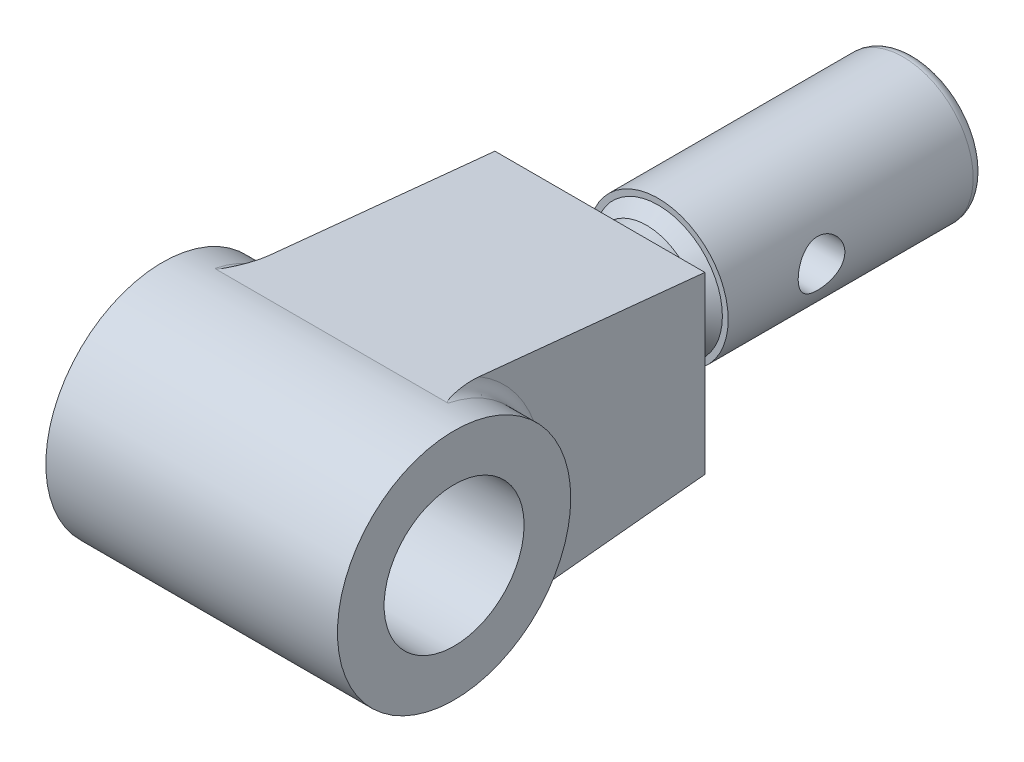
ISO-10303-21;
HEADER;
FILE_DESCRIPTION(('STEP AP214'),'2;1');
FILE_NAME('part.step','',(''),(''),'','','');
FILE_SCHEMA(('AUTOMOTIVE_DESIGN { 1 0 10303 214 1 1 1 1 }'));
ENDSEC;
DATA;
#1=APPLICATION_CONTEXT('core data for automotive mechanical design processes');
#2=APPLICATION_PROTOCOL_DEFINITION('international standard','automotive_design',2000,#1);
#3=PRODUCT_CONTEXT('',#1,'mechanical');
#4=PRODUCT('Part','Part','',(#3));
#5=PRODUCT_RELATED_PRODUCT_CATEGORY('part','',(#4));
#6=PRODUCT_DEFINITION_FORMATION('','',#4);
#7=PRODUCT_DEFINITION_CONTEXT('part definition',#1,'design');
#8=PRODUCT_DEFINITION('design','',#6,#7);
#9=PRODUCT_DEFINITION_SHAPE('','',#8);
#10=(LENGTH_UNIT() NAMED_UNIT(*) SI_UNIT(.MILLI.,.METRE.));
#11=(NAMED_UNIT(*) PLANE_ANGLE_UNIT() SI_UNIT($,.RADIAN.));
#12=(NAMED_UNIT(*) SI_UNIT($,.STERADIAN.) SOLID_ANGLE_UNIT());
#13=UNCERTAINTY_MEASURE_WITH_UNIT(LENGTH_MEASURE(1.E-05),#10,'distance_accuracy_value','');
#14=(GEOMETRIC_REPRESENTATION_CONTEXT(3) GLOBAL_UNCERTAINTY_ASSIGNED_CONTEXT((#13)) GLOBAL_UNIT_ASSIGNED_CONTEXT((#10,
#11,#12)) REPRESENTATION_CONTEXT('',''));
#15=CARTESIAN_POINT('',(0.,0.,0.));
#16=DIRECTION('',(0.,0.,1.));
#17=DIRECTION('',(1.,0.,0.));
#18=AXIS2_PLACEMENT_3D('',#15,#16,#17);
#19=CARTESIAN_POINT('',(0.,4.75247524752475,-0.475247524752475));
#20=DIRECTION('',(0.,0.995037190209989,-0.0995037190209989));
#21=DIRECTION('',(0.,0.0995037190209989,0.995037190209989));
#22=AXIS2_PLACEMENT_3D('',#19,#20,#21);
#23=PLANE('',#22);
#24=DIRECTION('',(0.,-0.0995037190209989,-0.995037190209989));
#25=VECTOR('',#24,1.);
#26=CARTESIAN_POINT('',(-9.,10.,52.));
#27=LINE('',#26,#25);
#28=CARTESIAN_POINT('',(-9.,9.43438132008126,46.3438132008126));
#29=VERTEX_POINT('',#28);
#30=CARTESIAN_POINT('',(-9.,7.5,27.));
#31=VERTEX_POINT('',#30);
#32=EDGE_CURVE('E120',#29,#31,#27,.T.);
#33=ORIENTED_EDGE('',*,*,#32,.F.);
#34=CARTESIAN_POINT('',(-9.,9.43438132008126,46.3438132008126));
#35=CARTESIAN_POINT('',(-9.00001459803866,9.44279857819186,46.4279857819186));
#36=CARTESIAN_POINT('',(-9.00195007259903,9.45121395233566,46.5121395233566));
#37=CARTESIAN_POINT('',(-9.00925721243809,9.46802699368894,46.6802699368894));
#38=CARTESIAN_POINT('',(-9.01462757621855,9.47642466639695,46.7642466639695));
#39=CARTESIAN_POINT('',(-9.02839065402064,9.4931839174512,46.931839174512));
#40=CARTESIAN_POINT('',(-9.03677945197559,9.50154552842399,47.0154552842398));
#41=CARTESIAN_POINT('',(-9.05626603490288,9.51823793957924,47.1823793957924));
#42=CARTESIAN_POINT('',(-9.06736410968055,9.52656873636875,47.2656873636875));
#43=CARTESIAN_POINT('',(-9.1042239175738,9.55145319834917,47.5145319834917));
#44=CARTESIAN_POINT('',(-9.13360055531106,9.5679543693951,47.679543693951));
#45=CARTESIAN_POINT('',(-9.20036560076197,9.60079627564721,48.0079627564722));
#46=CARTESIAN_POINT('',(-9.23775582627735,9.61713697357066,48.1713697357066));
#47=CARTESIAN_POINT('',(-9.30382525269167,9.64337755100343,48.4337755100343));
#48=CARTESIAN_POINT('',(-9.3303085460812,9.65333275535504,48.5333275535504));
#49=CARTESIAN_POINT('',(-9.38591969959388,9.6731705062701,48.7317050627009));
#50=CARTESIAN_POINT('',(-9.41504775619662,9.68305304737633,48.8305304737633));
#51=CARTESIAN_POINT('',(-9.4868107569843,9.70619439893835,49.0619439893834));
#52=CARTESIAN_POINT('',(-9.53059368398147,9.71941852182165,49.1941852182164));
#53=CARTESIAN_POINT('',(-9.6098255608624,9.74130040667283,49.4130040667283));
#54=CARTESIAN_POINT('',(-9.64327328731144,9.7500283022922,49.500283022922));
#55=CARTESIAN_POINT('',(-9.70409318445665,9.7644107399891,49.644107399891));
#56=CARTESIAN_POINT('',(-9.72984469495091,9.77013184956829,49.7013184956829));
#57=CARTESIAN_POINT('',(-9.77730952141487,9.77951878900499,49.7951878900499));
#58=CARTESIAN_POINT('',(-9.79763054155861,9.78325029234061,49.8325029234061));
#59=CARTESIAN_POINT('',(-9.83152593740173,9.788625396293,49.88625396293));
#60=CARTESIAN_POINT('',(-9.84336282293241,9.79037636611875,49.9037636611875));
#61=CARTESIAN_POINT('',(-9.86880656445889,9.79374682709678,49.9374682709678));
#62=CARTESIAN_POINT('',(-9.88240732968119,9.79536674089937,49.9536674089937));
#63=CARTESIAN_POINT('',(-9.90362979230834,9.7974453615268,49.974453615268));
#64=CARTESIAN_POINT('',(-9.91003887946058,9.79802485359438,49.9802485359437));
#65=CARTESIAN_POINT('',(-9.92347492697489,9.79911049653625,49.9911049653625));
#66=CARTESIAN_POINT('',(-9.93050194685285,9.79961664033359,49.9961664033359));
#67=CARTESIAN_POINT('',(-9.94390664000616,9.80043519672147,50.0043519672147));
#68=CARTESIAN_POINT('',(-9.95016816320597,9.80076611032304,50.0076611032304));
#69=CARTESIAN_POINT('',(-9.96313447059713,9.80132304768613,50.0132304768613));
#70=CARTESIAN_POINT('',(-9.96983721587579,9.80154951986671,50.015495198667));
#71=CARTESIAN_POINT('',(-9.98050267325267,9.80179749812321,50.017974981232));
#72=CARTESIAN_POINT('',(-9.98435828622742,9.8018653659966,50.018653659966));
#73=CARTESIAN_POINT('',(-9.99214094724413,9.80195700184466,50.0195700184466));
#74=CARTESIAN_POINT('',(-9.99606825420468,9.80198055014812,50.0198055014812));
#75=CARTESIAN_POINT('',(-10.0000000000001,9.80198019801976,50.0198019801975));
#76=B_SPLINE_CURVE_WITH_KNOTS('',3,(#34,#35,#36,#37,#38,#39,#40,#41,#42,#43,#44,#45,#46,#47,#48,
#49,#50,#51,#52,#53,#54,#55,#56,#57,#58,#59,#60,#61,#62,#63,#64,#65,#66,#67,#68,#69,#70,#71,#72,
#73,#74,#75),.UNSPECIFIED.,.F.,.F.,(4,2,2,2,2,2,2,2,2,2,2,2,2,2,2,2,2,2,2,2,4),(0.,
0.253728248763544,0.50736041542031,0.760664703401632,1.0139960986604,1.51898381324695,
2.02408620068496,2.33453599252592,2.64500886659734,3.06465085368098,3.34614880138818,
3.53504977951506,3.66278598087976,3.72636749640768,3.78973503293948,3.81567904004432,
3.8416255486758,3.86282853734113,3.88393962347977,3.89566215237055,3.90744263283122),.UNSPECIFIED.);
#77=CARTESIAN_POINT('',(-10.,9.80198019801981,50.0198019801981));
#78=VERTEX_POINT('',#77);
#79=EDGE_CURVE('E199',#29,#78,#76,.T.);
#80=ORIENTED_EDGE('',*,*,#79,.T.);
#81=DIRECTION('',(-1.,0.,0.));
#82=VECTOR('',#81,1.);
#83=CARTESIAN_POINT('',(12.5,9.80198019801981,50.0198019801981));
#84=LINE('',#83,#82);
#85=CARTESIAN_POINT('',(10.,9.80198019801981,50.0198019801981));
#86=VERTEX_POINT('',#85);
#87=EDGE_CURVE('E301',#78,#86,#84,.F.);
#88=ORIENTED_EDGE('',*,*,#87,.T.);
#89=CARTESIAN_POINT('',(10.,9.80198019801981,50.0198019801981));
#90=CARTESIAN_POINT('',(9.99296283793337,9.8019830885568,50.0198308855679));
#91=CARTESIAN_POINT('',(9.9859739614328,9.80190604043413,50.0190604043413));
#92=CARTESIAN_POINT('',(9.97240162965833,9.80162164853154,50.0162164853154));
#93=CARTESIAN_POINT('',(9.96581297534647,9.80141682642845,50.0141682642845));
#94=CARTESIAN_POINT('',(9.95111577822541,9.80082606313095,50.0082606313095));
#95=CARTESIAN_POINT('',(9.9431596448763,9.80040386580161,50.0040386580161));
#96=CARTESIAN_POINT('',(9.92794689579799,9.79944115886432,49.9944115886432));
#97=CARTESIAN_POINT('',(9.9206967876948,9.79889967585072,49.9889967585072));
#98=CARTESIAN_POINT('',(9.89592157562899,9.7968346648186,49.968346648186));
#99=CARTESIAN_POINT('',(9.88017272745921,9.79510616822487,49.9510616822487));
#100=CARTESIAN_POINT('',(9.85104447318803,9.79146606575537,49.9146606575537));
#101=CARTESIAN_POINT('',(9.83767936146509,9.78955345459827,49.8955345459827));
#102=CARTESIAN_POINT('',(9.81123761684502,9.78544512334652,49.8544512334651));
#103=CARTESIAN_POINT('',(9.79831048995985,9.78323981166724,49.8323981166724));
#104=CARTESIAN_POINT('',(9.77362495347973,9.77876478882271,49.7876478882271));
#105=CARTESIAN_POINT('',(9.76186765275939,9.77649501912824,49.7649501912824));
#106=CARTESIAN_POINT('',(9.72776607611959,9.76961556971392,49.6961556971392));
#107=CARTESIAN_POINT('',(9.70665112444375,9.7649457938296,49.649457938296));
#108=CARTESIAN_POINT('',(9.6662841980086,9.75551863142072,49.5551863142072));
#109=CARTESIAN_POINT('',(9.64703609746953,9.7507610861013,49.507610861013));
#110=CARTESIAN_POINT('',(9.60990653921663,9.741201996385,49.41201996385));
#111=CARTESIAN_POINT('',(9.59202302563084,9.73640053089024,49.3640053089024));
#112=CARTESIAN_POINT('',(9.53996928538504,9.7219691644136,49.219691644136));
#113=CARTESIAN_POINT('',(9.50728943722673,9.71228622272415,49.1228622272415));
#114=CARTESIAN_POINT('',(9.44483288869146,9.69282715969789,48.9282715969789));
#115=CARTESIAN_POINT('',(9.41505676766696,9.68305102019161,48.8305102019161));
#116=CARTESIAN_POINT('',(9.35808466058524,9.66341027274887,48.6341027274887));
#117=CARTESIAN_POINT('',(9.33089218385423,9.65354556385435,48.5354556385435));
#118=CARTESIAN_POINT('',(9.27911674500741,9.63374849171869,48.3374849171869));
#119=CARTESIAN_POINT('',(9.25453388737009,9.62381612578577,48.2381612578577));
#120=CARTESIAN_POINT('',(9.18510710789731,9.59401519656019,47.9401519656019));
#121=CARTESIAN_POINT('',(9.14431729261801,9.57405098307125,47.7405098307125));
#122=CARTESIAN_POINT('',(9.0759304674414,9.5339160612927,47.339160612927));
#123=CARTESIAN_POINT('',(9.04831757473376,9.51374563168741,47.1374563168741));
#124=CARTESIAN_POINT('',(9.01991153697103,9.48367802750643,46.8367802750643));
#125=CARTESIAN_POINT('',(9.01263009290031,9.47384138978838,46.7384138978838));
#126=CARTESIAN_POINT('',(9.00268266275587,9.45413163230314,46.5413163230314));
#127=CARTESIAN_POINT('',(9.00002319134237,9.44425848066686,46.4425848066686));
#128=CARTESIAN_POINT('',(9.,9.43438132008126,46.3438132008126));
#129=B_SPLINE_CURVE_WITH_KNOTS('',3,(#89,#90,#91,#92,#93,#94,#95,#96,#97,#98,#99,#100,#101,#102,
#103,#104,#105,#106,#107,#108,#109,#110,#111,#112,#113,#114,#115,#116,#117,#118,#119,#120,#121,
#122,#123,#124,#125,#126,#127,#128),.UNSPECIFIED.,.F.,.F.,(4,2,2,2,2,2,2,2,2,2,2,2,2,2,2,2,2,2,
2,4),(0.,0.0209921174012221,0.0415825099264115,0.0684781502878955,0.0956019813169603,
0.165390887755823,0.235585166584205,0.312484558399252,0.389456162026898,0.543749203982276,
0.698355885547646,0.852724840503093,1.16061515200922,1.46856676872982,1.77693086456379,
2.0853073013848,2.69918143578108,3.31231375591392,3.6095918243545,3.90728856677114),.UNSPECIFIED.);
#130=CARTESIAN_POINT('',(9.,9.43438132008126,46.3438132008126));
#131=VERTEX_POINT('',#130);
#132=EDGE_CURVE('E80',#86,#131,#129,.T.);
#133=ORIENTED_EDGE('',*,*,#132,.T.);
#134=DIRECTION('',(0.,-0.0995037190209989,-0.995037190209989));
#135=VECTOR('',#134,1.);
#136=CARTESIAN_POINT('',(9.,10.,52.));
#137=LINE('',#136,#135);
#138=CARTESIAN_POINT('',(9.,7.5,27.));
#139=VERTEX_POINT('',#138);
#140=EDGE_CURVE('E285',#131,#139,#137,.T.);
#141=ORIENTED_EDGE('',*,*,#140,.T.);
#142=DIRECTION('',(-1.,0.,0.));
#143=VECTOR('',#142,1.);
#144=CARTESIAN_POINT('',(-9.,7.5,27.));
#145=LINE('',#144,#143);
#146=EDGE_CURVE('E133',#139,#31,#145,.T.);
#147=ORIENTED_EDGE('',*,*,#146,.T.);
#148=EDGE_LOOP('',(#33,#80,#88,#133,#141,#147));
#149=FACE_BOUND('',#148,.T.);
#150=ADVANCED_FACE('F52',(#149),#23,.T.);
#151=CARTESIAN_POINT('',(0.,-4.75247524752475,-0.475247524752475));
#152=DIRECTION('',(0.,-0.995037190209989,-0.0995037190209989));
#153=DIRECTION('',(0.,0.0995037190209989,-0.995037190209989));
#154=AXIS2_PLACEMENT_3D('',#151,#152,#153);
#155=PLANE('',#154);
#156=DIRECTION('',(0.,0.0995037190209989,-0.995037190209989));
#157=VECTOR('',#156,1.);
#158=CARTESIAN_POINT('',(9.,-10.,52.));
#159=LINE('',#158,#157);
#160=CARTESIAN_POINT('',(9.,-9.43438132008126,46.3438132008126));
#161=VERTEX_POINT('',#160);
#162=CARTESIAN_POINT('',(9.,-7.5,27.));
#163=VERTEX_POINT('',#162);
#164=EDGE_CURVE('E107',#161,#163,#159,.T.);
#165=ORIENTED_EDGE('',*,*,#164,.F.);
#166=CARTESIAN_POINT('',(9.,-9.43438132008126,46.3438132008126));
#167=CARTESIAN_POINT('',(9.00001459803866,-9.44279857819186,46.4279857819186));
#168=CARTESIAN_POINT('',(9.00195007259902,-9.45121395233566,46.5121395233566));
#169=CARTESIAN_POINT('',(9.00925721243808,-9.46802699368894,46.6802699368894));
#170=CARTESIAN_POINT('',(9.01462757621855,-9.47642466639695,46.7642466639695));
#171=CARTESIAN_POINT('',(9.02839065402063,-9.4931839174512,46.931839174512));
#172=CARTESIAN_POINT('',(9.03677945197558,-9.50154552842398,47.0154552842398));
#173=CARTESIAN_POINT('',(9.05626603490288,-9.51823793957924,47.1823793957924));
#174=CARTESIAN_POINT('',(9.06736410968054,-9.52656873636875,47.2656873636875));
#175=CARTESIAN_POINT('',(9.1042239175738,-9.55145319834917,47.5145319834917));
#176=CARTESIAN_POINT('',(9.13360055531106,-9.5679543693951,47.679543693951));
#177=CARTESIAN_POINT('',(9.20036560076196,-9.60079627564721,48.0079627564722));
#178=CARTESIAN_POINT('',(9.23775582627735,-9.61713697357066,48.1713697357066));
#179=CARTESIAN_POINT('',(9.30382525269166,-9.64337755100343,48.4337755100343));
#180=CARTESIAN_POINT('',(9.3303085460812,-9.65333275535504,48.5333275535504));
#181=CARTESIAN_POINT('',(9.38591969959388,-9.6731705062701,48.7317050627009));
#182=CARTESIAN_POINT('',(9.41504775619661,-9.68305304737634,48.8305304737633));
#183=CARTESIAN_POINT('',(9.4868107569843,-9.70619439893835,49.0619439893834));
#184=CARTESIAN_POINT('',(9.53059368398148,-9.71941852182164,49.1941852182165));
#185=CARTESIAN_POINT('',(9.6098255608624,-9.74130040667283,49.4130040667283));
#186=CARTESIAN_POINT('',(9.64327328731144,-9.75002830229221,49.5002830229221));
#187=CARTESIAN_POINT('',(9.70409318445665,-9.7644107399891,49.644107399891));
#188=CARTESIAN_POINT('',(9.72984469495092,-9.77013184956829,49.7013184956829));
#189=CARTESIAN_POINT('',(9.77730952141486,-9.77951878900499,49.7951878900499));
#190=CARTESIAN_POINT('',(9.79763054155859,-9.78325029234062,49.8325029234061));
#191=CARTESIAN_POINT('',(9.83152593740171,-9.788625396293,49.88625396293));
#192=CARTESIAN_POINT('',(9.84336282293241,-9.79037636611875,49.9037636611875));
#193=CARTESIAN_POINT('',(9.86880656445889,-9.79374682709678,49.9374682709678));
#194=CARTESIAN_POINT('',(9.88240732968116,-9.79536674089937,49.9536674089937));
#195=CARTESIAN_POINT('',(9.90362979230833,-9.79744536152681,49.9744536152681));
#196=CARTESIAN_POINT('',(9.91003887946057,-9.79802485359438,49.9802485359437));
#197=CARTESIAN_POINT('',(9.92347492697489,-9.79911049653625,49.9911049653624));
#198=CARTESIAN_POINT('',(9.93050194685284,-9.79961664033359,49.9961664033359));
#199=CARTESIAN_POINT('',(9.94390664000615,-9.80043519672147,50.0043519672147));
#200=CARTESIAN_POINT('',(9.95016816320596,-9.80076611032304,50.0076611032304));
#201=CARTESIAN_POINT('',(9.96313447059712,-9.80132304768613,50.0132304768613));
#202=CARTESIAN_POINT('',(9.96983721587578,-9.80154951986671,50.015495198667));
#203=CARTESIAN_POINT('',(9.98050267325266,-9.80179749812321,50.017974981232));
#204=CARTESIAN_POINT('',(9.98435828622742,-9.8018653659966,50.018653659966));
#205=CARTESIAN_POINT('',(9.99214094724413,-9.80195700184466,50.0195700184465));
#206=CARTESIAN_POINT('',(9.99606825420468,-9.80198055014812,50.0198055014812));
#207=CARTESIAN_POINT('',(10.0000000000001,-9.80198019801976,50.0198019801975));
#208=B_SPLINE_CURVE_WITH_KNOTS('',3,(#166,#167,#168,#169,#170,#171,#172,#173,#174,#175,#176,
#177,#178,#179,#180,#181,#182,#183,#184,#185,#186,#187,#188,#189,#190,#191,#192,#193,#194,#195,
#196,#197,#198,#199,#200,#201,#202,#203,#204,#205,#206,#207),.UNSPECIFIED.,.F.,.F.,(4,2,2,2,2,2,
2,2,2,2,2,2,2,2,2,2,2,2,2,2,4),(0.,0.253728248763537,0.507360415420296,0.760664703401617,
1.01399609866039,1.51898381324695,2.02408620068496,2.33453599252592,2.64500886659734,
3.064650853681,3.34614880138819,3.53504977951505,3.66278598087975,3.72636749640768,
3.78973503293948,3.81567904004432,3.84162554867579,3.86282853734113,3.88393962347977,
3.89566215237055,3.90744263283123),.UNSPECIFIED.);
#209=CARTESIAN_POINT('',(10.,-9.80198019801981,50.0198019801981));
#210=VERTEX_POINT('',#209);
#211=EDGE_CURVE('E70',#161,#210,#208,.T.);
#212=ORIENTED_EDGE('',*,*,#211,.T.);
#213=DIRECTION('',(-1.,0.,0.));
#214=VECTOR('',#213,1.);
#215=CARTESIAN_POINT('',(12.5,-9.80198019801981,50.0198019801981));
#216=LINE('',#215,#214);
#217=CARTESIAN_POINT('',(-10.,-9.80198019801981,50.0198019801981));
#218=VERTEX_POINT('',#217);
#219=EDGE_CURVE('E149',#210,#218,#216,.T.);
#220=ORIENTED_EDGE('',*,*,#219,.T.);
#221=CARTESIAN_POINT('',(-10.,-9.80198019801981,50.0198019801981));
#222=CARTESIAN_POINT('',(-9.99296283793337,-9.8019830885568,50.0198308855679));
#223=CARTESIAN_POINT('',(-9.9859739614328,-9.80190604043413,50.0190604043413));
#224=CARTESIAN_POINT('',(-9.97240162965832,-9.80162164853154,50.0162164853154));
#225=CARTESIAN_POINT('',(-9.96581297534646,-9.80141682642845,50.0141682642845));
#226=CARTESIAN_POINT('',(-9.95111577822541,-9.80082606313095,50.0082606313095));
#227=CARTESIAN_POINT('',(-9.9431596448763,-9.80040386580161,50.0040386580161));
#228=CARTESIAN_POINT('',(-9.92794689579798,-9.79944115886432,49.9944115886432));
#229=CARTESIAN_POINT('',(-9.92069678769479,-9.79889967585072,49.9889967585072));
#230=CARTESIAN_POINT('',(-9.89592157562899,-9.7968346648186,49.968346648186));
#231=CARTESIAN_POINT('',(-9.88017272745921,-9.79510616822487,49.9510616822487));
#232=CARTESIAN_POINT('',(-9.85104447318803,-9.79146606575537,49.9146606575537));
#233=CARTESIAN_POINT('',(-9.83767936146509,-9.78955345459827,49.8955345459827));
#234=CARTESIAN_POINT('',(-9.81123761684502,-9.78544512334652,49.8544512334651));
#235=CARTESIAN_POINT('',(-9.79831048995985,-9.78323981166724,49.8323981166724));
#236=CARTESIAN_POINT('',(-9.77362495347973,-9.77876478882271,49.7876478882271));
#237=CARTESIAN_POINT('',(-9.76186765275939,-9.77649501912824,49.7649501912824));
#238=CARTESIAN_POINT('',(-9.72776607611958,-9.76961556971392,49.6961556971392));
#239=CARTESIAN_POINT('',(-9.70665112444375,-9.7649457938296,49.649457938296));
#240=CARTESIAN_POINT('',(-9.6662841980086,-9.75551863142072,49.5551863142072));
#241=CARTESIAN_POINT('',(-9.64703609746954,-9.7507610861013,49.507610861013));
#242=CARTESIAN_POINT('',(-9.60990653921663,-9.741201996385,49.41201996385));
#243=CARTESIAN_POINT('',(-9.59202302563084,-9.73640053089024,49.3640053089024));
#244=CARTESIAN_POINT('',(-9.53996928538504,-9.72196916441361,49.2196916441361));
#245=CARTESIAN_POINT('',(-9.50728943722674,-9.71228622272416,49.1228622272416));
#246=CARTESIAN_POINT('',(-9.44483288869147,-9.69282715969789,48.9282715969789));
#247=CARTESIAN_POINT('',(-9.41505676766696,-9.68305102019161,48.8305102019161));
#248=CARTESIAN_POINT('',(-9.35808466058525,-9.66341027274888,48.6341027274887));
#249=CARTESIAN_POINT('',(-9.33089218385424,-9.65354556385436,48.5354556385435));
#250=CARTESIAN_POINT('',(-9.27911674500742,-9.6337484917187,48.3374849171869));
#251=CARTESIAN_POINT('',(-9.2545338873701,-9.62381612578577,48.2381612578577));
#252=CARTESIAN_POINT('',(-9.18510710789733,-9.5940151965602,47.940151965602));
#253=CARTESIAN_POINT('',(-9.14431729261802,-9.57405098307126,47.7405098307126));
#254=CARTESIAN_POINT('',(-9.07593046744141,-9.53391606129271,47.3391606129271));
#255=CARTESIAN_POINT('',(-9.04831757473377,-9.51374563168741,47.1374563168741));
#256=CARTESIAN_POINT('',(-9.01991153697103,-9.48367802750644,46.8367802750644));
#257=CARTESIAN_POINT('',(-9.01263009290031,-9.47384138978839,46.7384138978839));
#258=CARTESIAN_POINT('',(-9.00268266275587,-9.45413163230314,46.5413163230314));
#259=CARTESIAN_POINT('',(-9.00002319134237,-9.44425848066686,46.4425848066686));
#260=CARTESIAN_POINT('',(-9.,-9.43438132008126,46.3438132008126));
#261=B_SPLINE_CURVE_WITH_KNOTS('',3,(#221,#222,#223,#224,#225,#226,#227,#228,#229,#230,#231,
#232,#233,#234,#235,#236,#237,#238,#239,#240,#241,#242,#243,#244,#245,#246,#247,#248,#249,#250,
#251,#252,#253,#254,#255,#256,#257,#258,#259,#260),.UNSPECIFIED.,.F.,.F.,(4,2,2,2,2,2,2,2,2,2,2,
2,2,2,2,2,2,2,2,4),(0.,0.0209921174012221,0.0415825099264115,0.0684781502878987,
0.0956019813169593,0.16539088775582,0.235585166584204,0.31248455839925,0.389456162026897,
0.543749203982268,0.698355885547638,0.852724840503072,1.1606151520092,1.46856676872979,
1.77693086456375,2.08530730138475,2.69918143578101,3.31231375591383,3.60959182435446,
3.90728856677114),.UNSPECIFIED.);
#262=CARTESIAN_POINT('',(-9.,-9.43438132008126,46.3438132008126));
#263=VERTEX_POINT('',#262);
#264=EDGE_CURVE('E280',#218,#263,#261,.T.);
#265=ORIENTED_EDGE('',*,*,#264,.T.);
#266=DIRECTION('',(0.,0.0995037190209989,-0.995037190209989));
#267=VECTOR('',#266,1.);
#268=CARTESIAN_POINT('',(-9.,-10.,52.));
#269=LINE('',#268,#267);
#270=CARTESIAN_POINT('',(-9.,-7.5,27.));
#271=VERTEX_POINT('',#270);
#272=EDGE_CURVE('E116',#263,#271,#269,.T.);
#273=ORIENTED_EDGE('',*,*,#272,.T.);
#274=DIRECTION('',(1.,0.,0.));
#275=VECTOR('',#274,1.);
#276=CARTESIAN_POINT('',(-9.,-7.5,27.));
#277=LINE('',#276,#275);
#278=EDGE_CURVE('E119',#271,#163,#277,.T.);
#279=ORIENTED_EDGE('',*,*,#278,.T.);
#280=EDGE_LOOP('',(#165,#212,#220,#265,#273,#279));
#281=FACE_BOUND('',#280,.T.);
#282=ADVANCED_FACE('F122',(#281),#155,.T.);
#283=CARTESIAN_POINT('',(0.,0.,27.));
#284=DIRECTION('',(0.,0.,-1.));
#285=DIRECTION('',(-1.,0.,0.));
#286=AXIS2_PLACEMENT_3D('',#283,#284,#285);
#287=CYLINDRICAL_SURFACE('',#286,6.);
#288=CARTESIAN_POINT('',(0.,0.,1.));
#289=DIRECTION('',(0.,0.,1.));
#290=DIRECTION('',(1.,0.,0.));
#291=AXIS2_PLACEMENT_3D('',#288,#289,#290);
#292=CIRCLE('',#291,6.);
#293=CARTESIAN_POINT('',(6.,0.,1.));
#294=VERTEX_POINT('',#293);
#295=EDGE_CURVE('E273',#294,#294,#292,.T.);
#296=ORIENTED_EDGE('',*,*,#295,.T.);
#297=EDGE_LOOP('',(#296));
#298=FACE_BOUND('',#297,.T.);
#299=CARTESIAN_POINT('',(-6.,0.,16.));
#300=CARTESIAN_POINT('',(-6.00000030601888,-0.109126725773446,16.0000005074633));
#301=CARTESIAN_POINT('',(-5.9969953901509,-0.2182503890771,15.9910394677456));
#302=CARTESIAN_POINT('',(-5.98530420406562,-0.433283521745944,15.9555417823656));
#303=CARTESIAN_POINT('',(-5.97661734404305,-0.539192656237636,15.9290033121022));
#304=CARTESIAN_POINT('',(-5.95450615812885,-0.744665579003552,15.8593615132319));
#305=CARTESIAN_POINT('',(-5.94108975461707,-0.844239651772068,15.8162858750815));
#306=CARTESIAN_POINT('',(-5.91088891434684,-1.03474987361065,15.7149176543233));
#307=CARTESIAN_POINT('',(-5.89410381335556,-1.12568431391741,15.6566220699948));
#308=CARTESIAN_POINT('',(-5.8582818888601,-1.29948335004453,15.5243483902825));
#309=CARTESIAN_POINT('',(-5.8391911292757,-1.38200740059662,15.449937531479));
#310=CARTESIAN_POINT('',(-5.80120629566243,-1.53366538540417,15.2884656905869));
#311=CARTESIAN_POINT('',(-5.78231226581098,-1.60279637097893,15.201401930143));
#312=CARTESIAN_POINT('',(-5.74626664954548,-1.72764988445572,15.0140297696071));
#313=CARTESIAN_POINT('',(-5.72918078551376,-1.78292971644206,14.9134125205358));
#314=CARTESIAN_POINT('',(-5.69950610837202,-1.87563774775544,14.7036478110829));
#315=CARTESIAN_POINT('',(-5.68691592321491,-1.91307139477353,14.5945029656745));
#316=CARTESIAN_POINT('',(-5.66822606538755,-1.96774692301833,14.3746535570066));
#317=CARTESIAN_POINT('',(-5.66192191539223,-1.98562689654354,14.2641255830219));
#318=CARTESIAN_POINT('',(-5.65591313259015,-2.00268224666895,14.0414724916882));
#319=CARTESIAN_POINT('',(-5.6562064604546,-2.00186340320944,13.9293478785816));
#320=CARTESIAN_POINT('',(-5.6631803001636,-1.98203980740684,13.712126739112));
#321=CARTESIAN_POINT('',(-5.66956831735066,-1.96386782633399,13.606943194162));
#322=CARTESIAN_POINT('',(-5.68753315449102,-1.91121232569883,13.4012131607863));
#323=CARTESIAN_POINT('',(-5.69911059568215,-1.87672685318374,13.3006672291299));
#324=CARTESIAN_POINT('',(-5.72635822262498,-1.79187811612042,13.105174500817));
#325=CARTESIAN_POINT('',(-5.74209131586235,-1.74126809741453,13.0103439490609));
#326=CARTESIAN_POINT('',(-5.77585117151453,-1.62577821260628,12.8302581834406));
#327=CARTESIAN_POINT('',(-5.79387859580927,-1.56089422472801,12.7450057461332));
#328=CARTESIAN_POINT('',(-5.83134658335482,-1.41469866536447,12.5818168036785));
#329=CARTESIAN_POINT('',(-5.85081178709686,-1.33270630015262,12.5044946109819));
#330=CARTESIAN_POINT('',(-5.88813876774073,-1.15667913994013,12.3645374666732));
#331=CARTESIAN_POINT('',(-5.90600039076135,-1.06264319132163,12.301903923671));
#332=CARTESIAN_POINT('',(-5.93834215875587,-0.863895226092535,12.1926073995299));
#333=CARTESIAN_POINT('',(-5.95278700016078,-0.759086552832672,12.1461090173185));
#334=CARTESIAN_POINT('',(-5.9764113428887,-0.542538166729014,12.0715936520886));
#335=CARTESIAN_POINT('',(-5.98559267309759,-0.430800876309907,12.0435702491531));
#336=CARTESIAN_POINT('',(-5.99735254142881,-0.208767659058608,12.0078886679553));
#337=CARTESIAN_POINT('',(-6.00020003667456,-0.0986191997296921,11.9994003816545));
#338=CARTESIAN_POINT('',(-5.99977805389655,0.121550139920475,12.0006653471969));
#339=CARTESIAN_POINT('',(-5.99650960838725,0.231571038639301,12.0104155199598));
#340=CARTESIAN_POINT('',(-5.98440049434209,0.445039732608511,12.0472238154719));
#341=CARTESIAN_POINT('',(-5.97572397422385,0.548585613669687,12.073772412099));
#342=CARTESIAN_POINT('',(-5.9538369366014,0.749711917159147,12.1427868889335));
#343=CARTESIAN_POINT('',(-5.9406258409335,0.847291577017213,12.1852547989356));
#344=CARTESIAN_POINT('',(-5.91057862574579,1.03657659278655,12.2861408636816));
#345=CARTESIAN_POINT('',(-5.89365629511572,1.12805991843429,12.3449491865663));
#346=CARTESIAN_POINT('',(-5.85810507832525,1.30012966027117,12.476388300027));
#347=CARTESIAN_POINT('',(-5.83947567187655,1.38071273559115,12.5490233120635));
#348=CARTESIAN_POINT('',(-5.8015369596089,1.5325050156126,12.7099575020132));
#349=CARTESIAN_POINT('',(-5.78223522174856,1.60312193849154,12.7988184538537));
#350=CARTESIAN_POINT('',(-5.74599946589417,1.72851504464715,12.9875431356218));
#351=CARTESIAN_POINT('',(-5.72906546764005,1.78329109586203,13.0874069572682));
#352=CARTESIAN_POINT('',(-5.69964783582767,1.87519386083272,13.2953460305798));
#353=CARTESIAN_POINT('',(-5.68715521585958,1.91235626433004,13.4034041583375));
#354=CARTESIAN_POINT('',(-5.66821664612899,1.96778933351871,13.6247573000883));
#355=CARTESIAN_POINT('',(-5.66176797247279,1.98606850990788,13.7380499308087));
#356=CARTESIAN_POINT('',(-5.65595717748355,2.00255256495468,13.9603941920818));
#357=CARTESIAN_POINT('',(-5.6562480051483,2.0017405146168,14.0693646805736));
#358=CARTESIAN_POINT('',(-5.66302539647735,1.98248458689739,14.2855301498441));
#359=CARTESIAN_POINT('',(-5.66951159138723,1.96404175891717,14.3927252359102));
#360=CARTESIAN_POINT('',(-5.68769048609783,1.91074362625869,14.6002713260049));
#361=CARTESIAN_POINT('',(-5.69928196044955,1.87620669203103,14.700713650009));
#362=CARTESIAN_POINT('',(-5.72632797636937,1.79195873151949,14.8944548138765));
#363=CARTESIAN_POINT('',(-5.74178337526786,1.74224433710761,14.987752062376));
#364=CARTESIAN_POINT('',(-5.77565658452093,1.62652138516686,15.1689673398458));
#365=CARTESIAN_POINT('',(-5.79417423284274,1.55989648552916,15.2564730037968));
#366=CARTESIAN_POINT('',(-5.83166712566506,1.4132857662713,15.4193796267684));
#367=CARTESIAN_POINT('',(-5.85064249824745,1.33329616890296,15.4947771513761));
#368=CARTESIAN_POINT('',(-5.88780061051088,1.15848311384137,15.6342888245784));
#369=CARTESIAN_POINT('',(-5.90592363602513,1.06320302699946,15.697848695502));
#370=CARTESIAN_POINT('',(-5.93851982345224,0.862714714813249,15.8079808577013));
#371=CARTESIAN_POINT('',(-5.9529939181586,0.757509036264697,15.8545574918441));
#372=CARTESIAN_POINT('',(-5.97611030137084,0.544987294401952,15.9274432649773));
#373=CARTESIAN_POINT('',(-5.98498424845045,0.437975515352818,15.9545649325268));
#374=CARTESIAN_POINT('',(-5.99692814128444,0.220640832020494,15.9908405613543));
#375=CARTESIAN_POINT('',(-5.9999996906381,0.110318851137493,15.9999994869931));
#376=CARTESIAN_POINT('',(-6.,0.,16.));
#377=B_SPLINE_CURVE_WITH_KNOTS('',3,(#299,#300,#301,#302,#303,#304,#305,#306,#307,#308,#309,
#310,#311,#312,#313,#314,#315,#316,#317,#318,#319,#320,#321,#322,#323,#324,#325,#326,#327,#328,
#329,#330,#331,#332,#333,#334,#335,#336,#337,#338,#339,#340,#341,#342,#343,#344,#345,#346,#347,
#348,#349,#350,#351,#352,#353,#354,#355,#356,#357,#358,#359,#360,#361,#362,#363,#364,#365,#366,
#367,#368,#369,#370,#371,#372,#373,#374,#375,#376),.UNSPECIFIED.,.T.,.F.,(4,2,2,2,2,2,2,2,2,2,2,
2,2,2,2,2,2,2,2,2,2,2,2,2,2,2,2,2,2,2,2,2,2,2,2,2,2,2,4),(0.,0.326974212052022,
0.653982370535041,0.980445345740546,1.3069727555982,1.64369368565512,1.98048866575061,
2.32696769646941,2.67334089385667,3.0080385148368,3.34263267974971,3.6619365310256,
3.98127861710964,4.30576342310261,4.63034205116414,4.97186611622734,5.31342291933237,
5.65836811300715,6.00319337754417,6.33307166350339,6.66289426328353,6.98316315956427,
7.30347290568208,7.63220799687473,7.96104361643782,8.30482045761504,8.64860016469993,
8.99168027653541,9.3346056941168,9.65991332128517,9.9852015870275,10.3043117416083,
10.6234927635196,10.9566013338361,11.2898042224756,11.635993216702,11.9820936230491,
12.3127311674763,12.6432773207628),.UNSPECIFIED.);
#378=CARTESIAN_POINT('',(-6.,0.,16.));
#379=VERTEX_POINT('',#378);
#380=EDGE_CURVE('E160',#379,#379,#377,.T.);
#381=ORIENTED_EDGE('',*,*,#380,.T.);
#382=EDGE_LOOP('',(#381));
#383=FACE_BOUND('',#382,.T.);
#384=CARTESIAN_POINT('',(6.,0.,12.));
#385=CARTESIAN_POINT('',(6.00000030601888,-0.109126725773446,11.9999994925367));
#386=CARTESIAN_POINT('',(5.9969953901509,-0.2182503890771,12.0089605322544));
#387=CARTESIAN_POINT('',(5.98530420406562,-0.433283521745944,12.0444582176344));
#388=CARTESIAN_POINT('',(5.97661734404305,-0.539192656237635,12.0709966878978));
#389=CARTESIAN_POINT('',(5.95450615812885,-0.744665579003553,12.1406384867681));
#390=CARTESIAN_POINT('',(5.94108975461707,-0.844239651772069,12.1837141249185));
#391=CARTESIAN_POINT('',(5.91088891434684,-1.03474987361065,12.2850823456767));
#392=CARTESIAN_POINT('',(5.89410381335556,-1.12568431391741,12.3433779300052));
#393=CARTESIAN_POINT('',(5.8582818888601,-1.29948335004453,12.4756516097175));
#394=CARTESIAN_POINT('',(5.8391911292757,-1.38200740059662,12.550062468521));
#395=CARTESIAN_POINT('',(5.80120629566243,-1.53366538540417,12.7115343094131));
#396=CARTESIAN_POINT('',(5.78231226581098,-1.60279637097892,12.798598069857));
#397=CARTESIAN_POINT('',(5.74626664954548,-1.72764988445572,12.9859702303929));
#398=CARTESIAN_POINT('',(5.72918078551376,-1.78292971644206,13.0865874794642));
#399=CARTESIAN_POINT('',(5.69950610837202,-1.87563774775544,13.2963521889171));
#400=CARTESIAN_POINT('',(5.68691592321491,-1.91307139477353,13.4054970343255));
#401=CARTESIAN_POINT('',(5.66822606538755,-1.96774692301833,13.6253464429934));
#402=CARTESIAN_POINT('',(5.66192191539223,-1.98562689654354,13.7358744169781));
#403=CARTESIAN_POINT('',(5.65591313259015,-2.00268224666895,13.9585275083118));
#404=CARTESIAN_POINT('',(5.6562064604546,-2.00186340320944,14.0706521214184));
#405=CARTESIAN_POINT('',(5.6631803001636,-1.98203980740684,14.287873260888));
#406=CARTESIAN_POINT('',(5.66956831735066,-1.96386782633399,14.393056805838));
#407=CARTESIAN_POINT('',(5.68753315449102,-1.91121232569883,14.5987868392137));
#408=CARTESIAN_POINT('',(5.69911059568215,-1.87672685318374,14.6993327708701));
#409=CARTESIAN_POINT('',(5.72635822262498,-1.79187811612042,14.894825499183));
#410=CARTESIAN_POINT('',(5.74209131586235,-1.74126809741453,14.9896560509391));
#411=CARTESIAN_POINT('',(5.77585117151453,-1.62577821260628,15.1697418165595));
#412=CARTESIAN_POINT('',(5.79387859580927,-1.56089422472801,15.2549942538668));
#413=CARTESIAN_POINT('',(5.83134658335482,-1.41469866536448,15.4181831963215));
#414=CARTESIAN_POINT('',(5.85081178709686,-1.33270630015262,15.4955053890181));
#415=CARTESIAN_POINT('',(5.88813876774073,-1.15667913994013,15.6354625333268));
#416=CARTESIAN_POINT('',(5.90600039076135,-1.06264319132163,15.698096076329));
#417=CARTESIAN_POINT('',(5.93834215875587,-0.863895226092535,15.8073926004701));
#418=CARTESIAN_POINT('',(5.95278700016078,-0.759086552832673,15.8538909826815));
#419=CARTESIAN_POINT('',(5.9764113428887,-0.542538166729014,15.9284063479114));
#420=CARTESIAN_POINT('',(5.98559267309759,-0.430800876309906,15.9564297508469));
#421=CARTESIAN_POINT('',(5.99735254142881,-0.208767659058607,15.9921113320447));
#422=CARTESIAN_POINT('',(6.00020003667456,-0.098619199729691,16.0005996183455));
#423=CARTESIAN_POINT('',(5.99977805389655,0.121550139920476,15.9993346528031));
#424=CARTESIAN_POINT('',(5.99650960838725,0.231571038639302,15.9895844800402));
#425=CARTESIAN_POINT('',(5.98440049434209,0.445039732608512,15.9527761845281));
#426=CARTESIAN_POINT('',(5.97572397422385,0.548585613669687,15.926227587901));
#427=CARTESIAN_POINT('',(5.9538369366014,0.749711917159147,15.8572131110665));
#428=CARTESIAN_POINT('',(5.9406258409335,0.847291577017213,15.8147452010644));
#429=CARTESIAN_POINT('',(5.91057862574579,1.03657659278655,15.7138591363184));
#430=CARTESIAN_POINT('',(5.89365629511572,1.12805991843429,15.6550508134337));
#431=CARTESIAN_POINT('',(5.85810507832525,1.30012966027117,15.523611699973));
#432=CARTESIAN_POINT('',(5.83947567187655,1.38071273559115,15.4509766879365));
#433=CARTESIAN_POINT('',(5.8015369596089,1.5325050156126,15.2900424979868));
#434=CARTESIAN_POINT('',(5.78223522174856,1.60312193849154,15.2011815461463));
#435=CARTESIAN_POINT('',(5.74599946589417,1.72851504464715,15.0124568643782));
#436=CARTESIAN_POINT('',(5.72906546764005,1.78329109586203,14.9125930427318));
#437=CARTESIAN_POINT('',(5.69964783582767,1.87519386083272,14.7046539694202));
#438=CARTESIAN_POINT('',(5.68715521585958,1.91235626433004,14.5965958416625));
#439=CARTESIAN_POINT('',(5.66821664612899,1.96778933351871,14.3752426999117));
#440=CARTESIAN_POINT('',(5.66176797247279,1.98606850990788,14.2619500691913));
#441=CARTESIAN_POINT('',(5.65595717748355,2.00255256495468,14.0396058079182));
#442=CARTESIAN_POINT('',(5.6562480051483,2.0017405146168,13.9306353194264));
#443=CARTESIAN_POINT('',(5.66302539647735,1.98248458689739,13.7144698501559));
#444=CARTESIAN_POINT('',(5.66951159138723,1.96404175891717,13.6072747640898));
#445=CARTESIAN_POINT('',(5.68769048609783,1.91074362625869,13.3997286739951));
#446=CARTESIAN_POINT('',(5.69928196044955,1.87620669203103,13.299286349991));
#447=CARTESIAN_POINT('',(5.72632797636937,1.79195873151949,13.1055451861235));
#448=CARTESIAN_POINT('',(5.74178337526786,1.74224433710761,13.012247937624));
#449=CARTESIAN_POINT('',(5.77565658452093,1.62652138516686,12.8310326601542));
#450=CARTESIAN_POINT('',(5.79417423284274,1.55989648552916,12.7435269962032));
#451=CARTESIAN_POINT('',(5.83166712566506,1.4132857662713,12.5806203732316));
#452=CARTESIAN_POINT('',(5.85064249824745,1.33329616890296,12.5052228486239));
#453=CARTESIAN_POINT('',(5.88780061051088,1.15848311384137,12.3657111754216));
#454=CARTESIAN_POINT('',(5.90592363602513,1.06320302699946,12.302151304498));
#455=CARTESIAN_POINT('',(5.93851982345224,0.862714714813248,12.1920191422987));
#456=CARTESIAN_POINT('',(5.9529939181586,0.757509036264696,12.1454425081559));
#457=CARTESIAN_POINT('',(5.97611030137084,0.544987294401951,12.0725567350227));
#458=CARTESIAN_POINT('',(5.98498424845045,0.437975515352817,12.0454350674732));
#459=CARTESIAN_POINT('',(5.99692814128444,0.220640832020494,12.0091594386457));
#460=CARTESIAN_POINT('',(5.9999996906381,0.110318851137493,12.0000005130069));
#461=CARTESIAN_POINT('',(6.,0.,12.));
#462=B_SPLINE_CURVE_WITH_KNOTS('',3,(#384,#385,#386,#387,#388,#389,#390,#391,#392,#393,#394,
#395,#396,#397,#398,#399,#400,#401,#402,#403,#404,#405,#406,#407,#408,#409,#410,#411,#412,#413,
#414,#415,#416,#417,#418,#419,#420,#421,#422,#423,#424,#425,#426,#427,#428,#429,#430,#431,#432,
#433,#434,#435,#436,#437,#438,#439,#440,#441,#442,#443,#444,#445,#446,#447,#448,#449,#450,#451,
#452,#453,#454,#455,#456,#457,#458,#459,#460,#461),.UNSPECIFIED.,.T.,.F.,(4,2,2,2,2,2,2,2,2,2,2,
2,2,2,2,2,2,2,2,2,2,2,2,2,2,2,2,2,2,2,2,2,2,2,2,2,2,2,4),(0.,0.326974212052022,
0.653982370535042,0.980445345740549,1.3069727555982,1.64369368565512,1.9804886657506,
2.32696769646941,2.67334089385667,3.0080385148368,3.34263267974971,3.6619365310256,
3.98127861710964,4.30576342310261,4.63034205116414,4.97186611622734,5.31342291933236,
5.65836811300715,6.00319337754417,6.33307166350339,6.66289426328353,6.98316315956427,
7.30347290568208,7.63220799687473,7.96104361643782,8.30482045761504,8.64860016469993,
8.99168027653541,9.3346056941168,9.65991332128517,9.9852015870275,10.3043117416084,
10.6234927635196,10.9566013338361,11.2898042224756,11.635993216702,11.9820936230491,
12.3127311674763,12.6432773207628),.UNSPECIFIED.);
#463=CARTESIAN_POINT('',(6.,0.,12.));
#464=VERTEX_POINT('',#463);
#465=EDGE_CURVE('E153',#464,#464,#462,.T.);
#466=ORIENTED_EDGE('',*,*,#465,.T.);
#467=EDGE_LOOP('',(#466));
#468=FACE_BOUND('',#467,.T.);
#469=CARTESIAN_POINT('',(0.,0.,22.));
#470=DIRECTION('',(0.,0.,1.));
#471=DIRECTION('',(1.,0.,0.));
#472=AXIS2_PLACEMENT_3D('',#469,#470,#471);
#473=CIRCLE('',#472,6.);
#474=CARTESIAN_POINT('',(6.,0.,22.));
#475=VERTEX_POINT('',#474);
#476=EDGE_CURVE('E138',#475,#475,#473,.T.);
#477=ORIENTED_EDGE('',*,*,#476,.F.);
#478=EDGE_LOOP('',(#477));
#479=FACE_BOUND('',#478,.T.);
#480=ADVANCED_FACE('F161',(#298,#383,#468,#479),#287,.T.);
#481=CARTESIAN_POINT('',(0.,0.,0.));
#482=DIRECTION('',(0.,0.,1.));
#483=DIRECTION('',(1.,0.,0.));
#484=AXIS2_PLACEMENT_3D('',#481,#482,#483);
#485=PLANE('',#484);
#486=CARTESIAN_POINT('',(0.,0.,0.));
#487=DIRECTION('',(0.,0.,1.));
#488=DIRECTION('',(1.,0.,0.));
#489=AXIS2_PLACEMENT_3D('',#486,#487,#488);
#490=CIRCLE('',#489,5.);
#491=CARTESIAN_POINT('',(5.,0.,0.));
#492=VERTEX_POINT('',#491);
#493=EDGE_CURVE('E274',#492,#492,#490,.F.);
#494=ORIENTED_EDGE('',*,*,#493,.T.);
#495=EDGE_LOOP('',(#494));
#496=FACE_BOUND('',#495,.T.);
#497=ADVANCED_FACE('F261',(#496),#485,.F.);
#498=CARTESIAN_POINT('',(0.,0.,27.000012));
#499=DIRECTION('',(0.,0.,-1.));
#500=DIRECTION('',(-1.,0.,0.));
#501=AXIS2_PLACEMENT_3D('',#498,#499,#500);
#502=CYLINDRICAL_SURFACE('',#501,4.5);
#503=CARTESIAN_POINT('',(0.,0.,23.));
#504=DIRECTION('',(0.,0.,1.));
#505=DIRECTION('',(1.,0.,0.));
#506=AXIS2_PLACEMENT_3D('',#503,#504,#505);
#507=CIRCLE('',#506,4.5);
#508=CARTESIAN_POINT('',(-4.5,0.,23.));
#509=VERTEX_POINT('',#508);
#510=EDGE_CURVE('E242',#509,#509,#507,.T.);
#511=CARTESIAN_POINT('',(0.,0.,26.));
#512=DIRECTION('',(0.,0.,1.));
#513=DIRECTION('',(1.,0.,0.));
#514=AXIS2_PLACEMENT_3D('',#511,#512,#513);
#515=CIRCLE('',#514,4.5);
#516=CARTESIAN_POINT('',(-4.5,0.,26.));
#517=VERTEX_POINT('',#516);
#518=EDGE_CURVE('E215',#517,#517,#515,.F.);
#519=CARTESIAN_POINT('',(-4.5,0.,23.));
#520=CARTESIAN_POINT('',(-4.5,0.,23.03125));
#521=CARTESIAN_POINT('',(-4.5,0.,23.0625));
#522=CARTESIAN_POINT('',(-4.5,0.,23.125));
#523=CARTESIAN_POINT('',(-4.5,0.,23.15625));
#524=CARTESIAN_POINT('',(-4.5,0.,23.21875));
#525=CARTESIAN_POINT('',(-4.5,0.,23.25));
#526=CARTESIAN_POINT('',(-4.5,0.,23.3125));
#527=CARTESIAN_POINT('',(-4.5,0.,23.34375));
#528=CARTESIAN_POINT('',(-4.5,0.,23.40625));
#529=CARTESIAN_POINT('',(-4.5,0.,23.4375));
#530=CARTESIAN_POINT('',(-4.5,0.,23.5));
#531=CARTESIAN_POINT('',(-4.5,0.,23.53125));
#532=CARTESIAN_POINT('',(-4.5,0.,23.59375));
#533=CARTESIAN_POINT('',(-4.5,0.,23.625));
#534=CARTESIAN_POINT('',(-4.5,0.,23.6875));
#535=CARTESIAN_POINT('',(-4.5,0.,23.71875));
#536=CARTESIAN_POINT('',(-4.5,0.,23.78125));
#537=CARTESIAN_POINT('',(-4.5,0.,23.8125));
#538=CARTESIAN_POINT('',(-4.5,0.,23.875));
#539=CARTESIAN_POINT('',(-4.5,0.,23.90625));
#540=CARTESIAN_POINT('',(-4.5,0.,23.96875));
#541=CARTESIAN_POINT('',(-4.5,0.,24.));
#542=CARTESIAN_POINT('',(-4.5,0.,24.0625));
#543=CARTESIAN_POINT('',(-4.5,0.,24.09375));
#544=CARTESIAN_POINT('',(-4.5,0.,24.15625));
#545=CARTESIAN_POINT('',(-4.5,0.,24.1875));
#546=CARTESIAN_POINT('',(-4.5,0.,24.25));
#547=CARTESIAN_POINT('',(-4.5,0.,24.28125));
#548=CARTESIAN_POINT('',(-4.5,0.,24.34375));
#549=CARTESIAN_POINT('',(-4.5,0.,24.375));
#550=CARTESIAN_POINT('',(-4.5,0.,24.4375));
#551=CARTESIAN_POINT('',(-4.5,0.,24.46875));
#552=CARTESIAN_POINT('',(-4.5,0.,24.53125));
#553=CARTESIAN_POINT('',(-4.5,0.,24.5625));
#554=CARTESIAN_POINT('',(-4.5,0.,24.625));
#555=CARTESIAN_POINT('',(-4.5,0.,24.65625));
#556=CARTESIAN_POINT('',(-4.5,0.,24.71875));
#557=CARTESIAN_POINT('',(-4.5,0.,24.75));
#558=CARTESIAN_POINT('',(-4.5,0.,24.8125));
#559=CARTESIAN_POINT('',(-4.5,0.,24.84375));
#560=CARTESIAN_POINT('',(-4.5,0.,24.90625));
#561=CARTESIAN_POINT('',(-4.5,0.,24.9375));
#562=CARTESIAN_POINT('',(-4.5,0.,25.));
#563=CARTESIAN_POINT('',(-4.5,0.,25.03125));
#564=CARTESIAN_POINT('',(-4.5,0.,25.09375));
#565=CARTESIAN_POINT('',(-4.5,0.,25.125));
#566=CARTESIAN_POINT('',(-4.5,0.,25.1875));
#567=CARTESIAN_POINT('',(-4.5,0.,25.21875));
#568=CARTESIAN_POINT('',(-4.5,0.,25.28125));
#569=CARTESIAN_POINT('',(-4.5,0.,25.3125));
#570=CARTESIAN_POINT('',(-4.5,0.,25.375));
#571=CARTESIAN_POINT('',(-4.5,0.,25.40625));
#572=CARTESIAN_POINT('',(-4.5,0.,25.46875));
#573=CARTESIAN_POINT('',(-4.5,0.,25.5));
#574=CARTESIAN_POINT('',(-4.5,0.,25.5625));
#575=CARTESIAN_POINT('',(-4.5,0.,25.59375));
#576=CARTESIAN_POINT('',(-4.5,0.,25.65625));
#577=CARTESIAN_POINT('',(-4.5,0.,25.6875));
#578=CARTESIAN_POINT('',(-4.5,0.,25.75));
#579=CARTESIAN_POINT('',(-4.5,0.,25.78125));
#580=CARTESIAN_POINT('',(-4.5,0.,25.84375));
#581=CARTESIAN_POINT('',(-4.5,0.,25.875));
#582=CARTESIAN_POINT('',(-4.5,0.,25.9375));
#583=CARTESIAN_POINT('',(-4.5,0.,25.96875));
#584=CARTESIAN_POINT('',(-4.5,0.,26.));
#585=B_SPLINE_CURVE_WITH_KNOTS('',3,(#519,#520,#521,#522,#523,#524,#525,#526,#527,#528,#529,
#530,#531,#532,#533,#534,#535,#536,#537,#538,#539,#540,#541,#542,#543,#544,#545,#546,#547,#548,
#549,#550,#551,#552,#553,#554,#555,#556,#557,#558,#559,#560,#561,#562,#563,#564,#565,#566,#567,
#568,#569,#570,#571,#572,#573,#574,#575,#576,#577,#578,#579,#580,#581,#582,#583,#584),
.UNSPECIFIED.,.F.,.F.,(4,2,2,2,2,2,2,2,2,2,2,2,2,2,2,2,2,2,2,2,2,2,2,2,2,2,2,2,2,2,2,2,4),(0.,
0.0937500000000001,0.187499999999997,0.281249999999997,0.374999999999993,0.468749999999993,
0.562499999999994,0.65624999999999,0.74999999999999,0.84374999999999,0.93749999999999,
1.03124999999999,1.12499999999999,1.21874999999999,1.31249999999998,1.40624999999998,
1.49999999999998,1.59374999999998,1.68749999999998,1.78124999999998,1.87499999999998,
1.96874999999998,2.06249999999998,2.15624999999997,2.24999999999997,2.34374999999997,
2.43749999999997,2.53124999999997,2.62499999999997,2.71874999999997,2.81249999999997,
2.90624999999997,2.99999999999997),.UNSPECIFIED.);
#586=EDGE_CURVE('BSEAM248',#509,#517,#585,.T.);
#587=ORIENTED_EDGE('',*,*,#510,.T.);
#588=ORIENTED_EDGE('',*,*,#518,.T.);
#589=ORIENTED_EDGE('',*,*,#586,.T.);
#590=ORIENTED_EDGE('',*,*,#586,.F.);
#591=EDGE_LOOP('',(#587,#589,#588,#590));
#592=FACE_BOUND('',#591,.T.);
#593=ADVANCED_FACE('F248',(#592),#502,.T.);
#594=CARTESIAN_POINT('',(0.,0.,22.));
#595=DIRECTION('',(0.,0.,1.));
#596=DIRECTION('',(1.,0.,0.));
#597=AXIS2_PLACEMENT_3D('',#594,#595,#596);
#598=PLANE('',#597);
#599=CARTESIAN_POINT('',(0.,0.,22.));
#600=DIRECTION('',(0.,0.,1.));
#601=DIRECTION('',(1.,0.,0.));
#602=AXIS2_PLACEMENT_3D('',#599,#600,#601);
#603=CIRCLE('',#602,5.50000000000002);
#604=CARTESIAN_POINT('',(5.50000000000002,0.,22.));
#605=VERTEX_POINT('',#604);
#606=EDGE_CURVE('E65',#605,#605,#603,.F.);
#607=ORIENTED_EDGE('',*,*,#606,.T.);
#608=EDGE_LOOP('',(#607));
#609=FACE_BOUND('',#608,.T.);
#610=ORIENTED_EDGE('',*,*,#476,.T.);
#611=EDGE_LOOP('',(#610));
#612=FACE_BOUND('',#611,.T.);
#613=ADVANCED_FACE('F254',(#609,#612),#598,.T.);
#614=CARTESIAN_POINT('',(0.,0.,27.));
#615=DIRECTION('',(0.,0.,1.));
#616=DIRECTION('',(1.,0.,0.));
#617=AXIS2_PLACEMENT_3D('',#614,#615,#616);
#618=PLANE('',#617);
#619=CARTESIAN_POINT('',(0.,0.,27.));
#620=DIRECTION('',(0.,0.,1.));
#621=DIRECTION('',(1.,0.,0.));
#622=AXIS2_PLACEMENT_3D('',#619,#620,#621);
#623=CIRCLE('',#622,5.50000000000002);
#624=CARTESIAN_POINT('',(5.50000000000002,0.,27.));
#625=VERTEX_POINT('',#624);
#626=EDGE_CURVE('E12',#625,#625,#623,.T.);
#627=ORIENTED_EDGE('',*,*,#626,.T.);
#628=EDGE_LOOP('',(#627));
#629=FACE_BOUND('',#628,.T.);
#630=DIRECTION('',(0.,1.,0.));
#631=VECTOR('',#630,1.);
#632=CARTESIAN_POINT('',(9.,7.5,27.));
#633=LINE('',#632,#631);
#634=EDGE_CURVE('E113',#163,#139,#633,.T.);
#635=ORIENTED_EDGE('',*,*,#634,.F.);
#636=ORIENTED_EDGE('',*,*,#278,.F.);
#637=DIRECTION('',(0.,-1.,0.));
#638=VECTOR('',#637,1.);
#639=CARTESIAN_POINT('',(-9.,7.5,27.));
#640=LINE('',#639,#638);
#641=EDGE_CURVE('E127',#31,#271,#640,.T.);
#642=ORIENTED_EDGE('',*,*,#641,.F.);
#643=ORIENTED_EDGE('',*,*,#146,.F.);
#644=EDGE_LOOP('',(#635,#636,#642,#643));
#645=FACE_BOUND('',#644,.T.);
#646=ADVANCED_FACE('F126',(#629,#645),#618,.F.);
#647=CARTESIAN_POINT('',(-9.,0.,0.));
#648=DIRECTION('',(-1.,0.,0.));
#649=DIRECTION('',(0.,-1.,0.));
#650=AXIS2_PLACEMENT_3D('',#647,#648,#649);
#651=PLANE('',#650);
#652=ORIENTED_EDGE('',*,*,#272,.F.);
#653=CARTESIAN_POINT('',(-9.,0.,52.));
#654=DIRECTION('',(-1.,0.,0.));
#655=DIRECTION('',(0.,-1.,0.));
#656=AXIS2_PLACEMENT_3D('',#653,#654,#655);
#657=CIRCLE('',#656,11.);
#658=EDGE_CURVE('E148',#263,#29,#657,.F.);
#659=ORIENTED_EDGE('',*,*,#658,.T.);
#660=ORIENTED_EDGE('',*,*,#32,.T.);
#661=ORIENTED_EDGE('',*,*,#641,.T.);
#662=EDGE_LOOP('',(#652,#659,#660,#661));
#663=FACE_BOUND('',#662,.T.);
#664=ADVANCED_FACE('F194',(#663),#651,.T.);
#665=CARTESIAN_POINT('',(9.,0.,0.));
#666=DIRECTION('',(1.,0.,0.));
#667=DIRECTION('',(0.,1.,0.));
#668=AXIS2_PLACEMENT_3D('',#665,#666,#667);
#669=PLANE('',#668);
#670=ORIENTED_EDGE('',*,*,#140,.F.);
#671=CARTESIAN_POINT('',(9.,0.,52.));
#672=DIRECTION('',(1.,0.,0.));
#673=DIRECTION('',(0.,1.,0.));
#674=AXIS2_PLACEMENT_3D('',#671,#672,#673);
#675=CIRCLE('',#674,11.);
#676=EDGE_CURVE('E112',#131,#161,#675,.F.);
#677=ORIENTED_EDGE('',*,*,#676,.T.);
#678=ORIENTED_EDGE('',*,*,#164,.T.);
#679=ORIENTED_EDGE('',*,*,#634,.T.);
#680=EDGE_LOOP('',(#670,#677,#678,#679));
#681=FACE_BOUND('',#680,.T.);
#682=ADVANCED_FACE('F111',(#681),#669,.T.);
#683=CARTESIAN_POINT('',(12.5,0.,52.));
#684=DIRECTION('',(1.,0.,0.));
#685=DIRECTION('',(0.,0.,-1.));
#686=AXIS2_PLACEMENT_3D('',#683,#684,#685);
#687=PLANE('',#686);
#688=CARTESIAN_POINT('',(12.5,0.,52.));
#689=DIRECTION('',(1.,0.,0.));
#690=DIRECTION('',(0.,0.,-1.));
#691=AXIS2_PLACEMENT_3D('',#688,#689,#690);
#692=CIRCLE('',#691,10.);
#693=CARTESIAN_POINT('',(12.5,0.,42.));
#694=VERTEX_POINT('',#693);
#695=EDGE_CURVE('E307',#694,#694,#692,.T.);
#696=ORIENTED_EDGE('',*,*,#695,.T.);
#697=EDGE_LOOP('',(#696));
#698=FACE_BOUND('',#697,.T.);
#699=CARTESIAN_POINT('',(12.5,0.,52.));
#700=DIRECTION('',(1.,0.,0.));
#701=DIRECTION('',(0.,0.,-1.));
#702=AXIS2_PLACEMENT_3D('',#699,#700,#701);
#703=CIRCLE('',#702,6.);
#704=CARTESIAN_POINT('',(12.5,0.,46.));
#705=VERTEX_POINT('',#704);
#706=EDGE_CURVE('E320',#705,#705,#703,.T.);
#707=ORIENTED_EDGE('',*,*,#706,.F.);
#708=EDGE_LOOP('',(#707));
#709=FACE_BOUND('',#708,.T.);
#710=ADVANCED_FACE('F177',(#698,#709),#687,.T.);
#711=CARTESIAN_POINT('',(-12.5,0.,52.));
#712=DIRECTION('',(1.,0.,0.));
#713=DIRECTION('',(0.,0.,-1.));
#714=AXIS2_PLACEMENT_3D('',#711,#712,#713);
#715=PLANE('',#714);
#716=CARTESIAN_POINT('',(-12.5,0.,52.));
#717=DIRECTION('',(1.,0.,0.));
#718=DIRECTION('',(0.,0.,-1.));
#719=AXIS2_PLACEMENT_3D('',#716,#717,#718);
#720=CIRCLE('',#719,10.);
#721=CARTESIAN_POINT('',(-12.5,0.,42.));
#722=VERTEX_POINT('',#721);
#723=EDGE_CURVE('E315',#722,#722,#720,.T.);
#724=ORIENTED_EDGE('',*,*,#723,.F.);
#725=EDGE_LOOP('',(#724));
#726=FACE_BOUND('',#725,.T.);
#727=CARTESIAN_POINT('',(-12.5,0.,52.));
#728=DIRECTION('',(1.,0.,0.));
#729=DIRECTION('',(0.,0.,-1.));
#730=AXIS2_PLACEMENT_3D('',#727,#728,#729);
#731=CIRCLE('',#730,6.);
#732=CARTESIAN_POINT('',(-12.5,0.,46.));
#733=VERTEX_POINT('',#732);
#734=EDGE_CURVE('E316',#733,#733,#731,.T.);
#735=ORIENTED_EDGE('',*,*,#734,.T.);
#736=EDGE_LOOP('',(#735));
#737=FACE_BOUND('',#736,.T.);
#738=ADVANCED_FACE('F185',(#726,#737),#715,.F.);
#739=CARTESIAN_POINT('',(12.5,0.,52.));
#740=DIRECTION('',(-1.,0.,0.));
#741=DIRECTION('',(0.,0.,1.));
#742=AXIS2_PLACEMENT_3D('',#739,#740,#741);
#743=CYLINDRICAL_SURFACE('',#742,10.);
#744=ORIENTED_EDGE('',*,*,#87,.F.);
#745=CARTESIAN_POINT('',(-10.,0.,52.));
#746=DIRECTION('',(-1.,0.,0.));
#747=DIRECTION('',(0.,-1.,0.));
#748=AXIS2_PLACEMENT_3D('',#745,#746,#747);
#749=CIRCLE('',#748,10.);
#750=EDGE_CURVE('E283',#78,#218,#749,.T.);
#751=ORIENTED_EDGE('',*,*,#750,.T.);
#752=ORIENTED_EDGE('',*,*,#219,.F.);
#753=CARTESIAN_POINT('',(10.,0.,52.));
#754=DIRECTION('',(1.,0.,0.));
#755=DIRECTION('',(0.,1.,0.));
#756=AXIS2_PLACEMENT_3D('',#753,#754,#755);
#757=CIRCLE('',#756,10.);
#758=EDGE_CURVE('E294',#210,#86,#757,.T.);
#759=ORIENTED_EDGE('',*,*,#758,.T.);
#760=EDGE_LOOP('',(#744,#751,#752,#759));
#761=FACE_BOUND('',#760,.T.);
#762=ORIENTED_EDGE('',*,*,#695,.F.);
#763=EDGE_LOOP('',(#762));
#764=FACE_BOUND('',#763,.T.);
#765=ORIENTED_EDGE('',*,*,#723,.T.);
#766=EDGE_LOOP('',(#765));
#767=FACE_BOUND('',#766,.T.);
#768=ADVANCED_FACE('F180',(#761,#764,#767),#743,.T.);
#769=CARTESIAN_POINT('',(12.5,0.,52.));
#770=DIRECTION('',(-1.,0.,0.));
#771=DIRECTION('',(0.,0.,1.));
#772=AXIS2_PLACEMENT_3D('',#769,#770,#771);
#773=CYLINDRICAL_SURFACE('',#772,6.);
#774=ORIENTED_EDGE('',*,*,#706,.T.);
#775=EDGE_LOOP('',(#774));
#776=FACE_BOUND('',#775,.T.);
#777=ORIENTED_EDGE('',*,*,#734,.F.);
#778=EDGE_LOOP('',(#777));
#779=FACE_BOUND('',#778,.T.);
#780=ADVANCED_FACE('F175',(#776,#779),#773,.F.);
#781=CARTESIAN_POINT('',(-12.5,0.,14.));
#782=DIRECTION('',(1.,0.,0.));
#783=DIRECTION('',(0.,0.,-1.));
#784=AXIS2_PLACEMENT_3D('',#781,#782,#783);
#785=CYLINDRICAL_SURFACE('',#784,2.);
#786=ORIENTED_EDGE('',*,*,#465,.F.);
#787=EDGE_LOOP('',(#786));
#788=FACE_BOUND('',#787,.T.);
#789=ORIENTED_EDGE('',*,*,#380,.F.);
#790=EDGE_LOOP('',(#789));
#791=FACE_BOUND('',#790,.T.);
#792=ADVANCED_FACE('F170',(#788,#791),#785,.F.);
#793=CARTESIAN_POINT('',(-10.,0.,52.));
#794=DIRECTION('',(-1.,0.,0.));
#795=DIRECTION('',(0.,-1.,0.));
#796=AXIS2_PLACEMENT_3D('',#793,#794,#795);
#797=TOROIDAL_SURFACE('',#796,11.,1.);
#798=ORIENTED_EDGE('',*,*,#264,.F.);
#799=ORIENTED_EDGE('',*,*,#750,.F.);
#800=ORIENTED_EDGE('',*,*,#79,.F.);
#801=ORIENTED_EDGE('',*,*,#658,.F.);
#802=EDGE_LOOP('',(#798,#799,#800,#801));
#803=FACE_BOUND('',#802,.T.);
#804=ADVANCED_FACE('F171',(#803),#797,.F.);
#805=CARTESIAN_POINT('',(10.,0.,52.));
#806=DIRECTION('',(1.,0.,0.));
#807=DIRECTION('',(0.,1.,0.));
#808=AXIS2_PLACEMENT_3D('',#805,#806,#807);
#809=TOROIDAL_SURFACE('',#808,11.,1.);
#810=ORIENTED_EDGE('',*,*,#132,.F.);
#811=ORIENTED_EDGE('',*,*,#758,.F.);
#812=ORIENTED_EDGE('',*,*,#211,.F.);
#813=ORIENTED_EDGE('',*,*,#676,.F.);
#814=EDGE_LOOP('',(#810,#811,#812,#813));
#815=FACE_BOUND('',#814,.T.);
#816=ADVANCED_FACE('F220',(#815),#809,.F.);
#817=CARTESIAN_POINT('',(0.,0.,1.));
#818=DIRECTION('',(0.,0.,1.));
#819=DIRECTION('',(1.,0.,0.));
#820=AXIS2_PLACEMENT_3D('',#817,#818,#819);
#821=TOROIDAL_SURFACE('',#820,5.,1.);
#822=ORIENTED_EDGE('',*,*,#493,.F.);
#823=EDGE_LOOP('',(#822));
#824=FACE_BOUND('',#823,.T.);
#825=ORIENTED_EDGE('',*,*,#295,.F.);
#826=EDGE_LOOP('',(#825));
#827=FACE_BOUND('',#826,.T.);
#828=ADVANCED_FACE('F222',(#824,#827),#821,.T.);
#829=CARTESIAN_POINT('',(0.,0.,23.));
#830=DIRECTION('',(0.,0.,-1.));
#831=DIRECTION('',(-1.,0.,0.));
#832=AXIS2_PLACEMENT_3D('',#829,#830,#831);
#833=CONICAL_SURFACE('',#832,4.5,0.785398163397445);
#834=ORIENTED_EDGE('',*,*,#606,.F.);
#835=EDGE_LOOP('',(#834));
#836=FACE_BOUND('',#835,.T.);
#837=ORIENTED_EDGE('',*,*,#510,.F.);
#838=EDGE_LOOP('',(#837));
#839=FACE_BOUND('',#838,.T.);
#840=ADVANCED_FACE('F227',(#836,#839),#833,.T.);
#841=CARTESIAN_POINT('',(0.,0.,27.));
#842=DIRECTION('',(0.,0.,1.));
#843=DIRECTION('',(1.,0.,0.));
#844=AXIS2_PLACEMENT_3D('',#841,#842,#843);
#845=CONICAL_SURFACE('',#844,5.50000000000002,0.785398163397453);
#846=ORIENTED_EDGE('',*,*,#518,.F.);
#847=EDGE_LOOP('',(#846));
#848=FACE_BOUND('',#847,.T.);
#849=ORIENTED_EDGE('',*,*,#626,.F.);
#850=EDGE_LOOP('',(#849));
#851=FACE_BOUND('',#850,.T.);
#852=ADVANCED_FACE('F57',(#848,#851),#845,.T.);
#853=CLOSED_SHELL('',(#150,#282,#480,#497,#593,#613,#646,#664,#682,#710,#738,#768,#780,#792,
#804,#816,#828,#840,#852));
#854=MANIFOLD_SOLID_BREP('B2',#853);
#855=ADVANCED_BREP_SHAPE_REPRESENTATION('',(#18,#854),#14);
#856=SHAPE_DEFINITION_REPRESENTATION(#9,#855);
ENDSEC;
END-ISO-10303-21;
